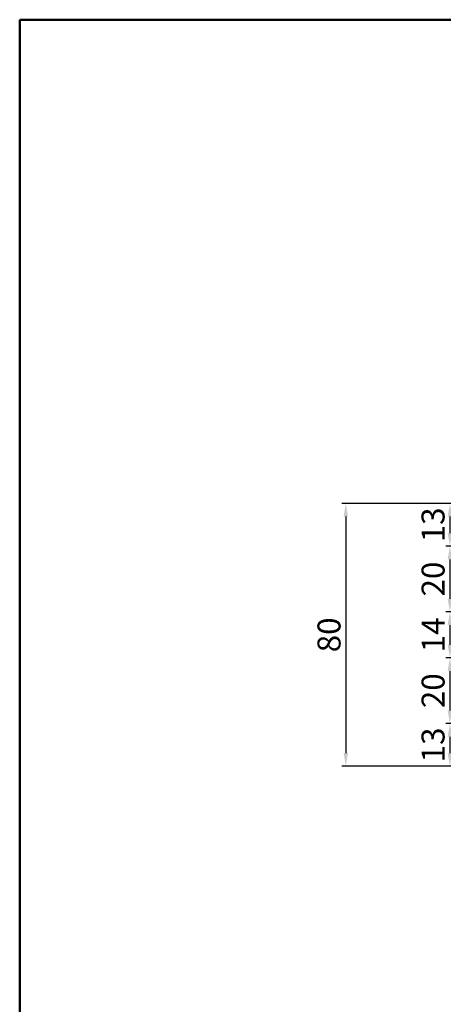
# Model space of a CAD drawing. Units: millimetres. Extents: x -21 to 693, y -570 to 295.
# Tile 3 of 7: x -21 to 107, y -4 to 295. Entities that reach past the tile are written whole.
import ezdxf

# ---------------------------------------------------------------- set-up
doc = ezdxf.new("R2010")
doc.units = ezdxf.units.MM
doc.header["$LTSCALE"] = 0.5
doc.layers.add('M-DIMS', color=2, linetype='Continuous', lineweight=25)
doc.layers.add('M-TTLB', color=7, linetype='Continuous', lineweight=50)
doc.styles.get("Standard").update_dxf_attribs({"font": 'arial.ttf'})
doc.dimstyles.new('ISO-25', dxfattribs={"dimtxt": 7, "dimasz": 4, "dimexe": 1.25, "dimexo": 0.625, "dimtad": 1, "dimdec": 0, "dimtxsty": 'Standard', "dimcen": 2.5, "dimadec": 0, "dimazin": 0, "dimtfac": 1, "dimtdec": 0, "dimtofl": 0, "dimtmove": 0, "dimatfit": 3, "dimfxl": 1, "dimarcsym": 0})

# ---------------------------------------------------------------- blocks, each defined once
blk = doc.blocks.new('*D6')
at = {"layer": 'Defpoints', "color": 0, "ltscale": 0.5, "transparency": 16777216}
for p in [(136.24, 148.11), (77.7, 68.11), (136.24, 68.11)]:
    blk.add_point(p, dxfattribs=at)
at = {"layer": 'M-DIMS', "color": 0, "lineweight": -2, "ltscale": 0.5, "transparency": 16777216}
for p, q in [((135.61, 148.11), (76.45, 148.11)), ((77.7, 144.11), (77.7, 72.11)), ((135.61, 68.11), (76.45, 68.11))]:
    blk.add_line(p, q, dxfattribs=at)
at = {"layer": 'M-DIMS', "color": 0, "ltscale": 0.5, "transparency": 16777216}
for points in [[(77.04, 144.11), (78.37, 144.11), (77.7, 148.11)], [(77.04, 72.11), (78.37, 72.11), (77.7, 68.11)]]:
    blk.add_solid(points, dxfattribs=at)
at = {"layer": 'M-DIMS', "color": 0, "ltscale": 0.5, "transparency": 16777216, "insert": (73.5, 108.11), "char_height": 7, "attachment_point": 5, "rotation": 90}
blk.add_mtext('80', dxfattribs=at)
blk = doc.blocks.new('*D7')
at = {"layer": 'Defpoints', "color": 0, "ltscale": 0.5, "transparency": 16777216}
for p in [(136.24, 148.11), (109.35, 135.11), (136.24, 135.11)]:
    blk.add_point(p, dxfattribs=at)
at = {"layer": 'M-DIMS', "color": 0, "lineweight": -2, "ltscale": 0.5, "transparency": 16777216}
for p, q in [((135.61, 148.11), (108.1, 148.11)), ((109.35, 144.11), (109.35, 139.11)), ((135.61, 135.11), (108.1, 135.11))]:
    blk.add_line(p, q, dxfattribs=at)
at = {"layer": 'M-DIMS', "color": 0, "ltscale": 0.5, "transparency": 16777216}
for points in [[(108.69, 144.11), (110.02, 144.11), (109.35, 148.11)], [(108.69, 139.11), (110.02, 139.11), (109.35, 135.11)]]:
    blk.add_solid(points, dxfattribs=at)
at = {"layer": 'M-DIMS', "color": 0, "ltscale": 0.5, "transparency": 16777216, "insert": (105.15, 141.61), "char_height": 7, "attachment_point": 5, "rotation": 90}
blk.add_mtext('13', dxfattribs=at)
blk = doc.blocks.new('*D8')
at = {"layer": 'Defpoints', "color": 0, "ltscale": 0.5, "transparency": 16777216}
for p in [(135.24, 135.11), (109.35, 115.11), (136.24, 115.11)]:
    blk.add_point(p, dxfattribs=at)
at = {"layer": 'M-DIMS', "color": 0, "lineweight": -2, "ltscale": 0.5, "transparency": 16777216}
for p, q in [((134.61, 135.11), (108.1, 135.11)), ((109.35, 131.11), (109.35, 119.11)), ((135.61, 115.11), (108.1, 115.11))]:
    blk.add_line(p, q, dxfattribs=at)
at = {"layer": 'M-DIMS', "color": 0, "ltscale": 0.5, "transparency": 16777216}
for points in [[(108.69, 131.11), (110.02, 131.11), (109.35, 135.11)], [(108.69, 119.11), (110.02, 119.11), (109.35, 115.11)]]:
    blk.add_solid(points, dxfattribs=at)
at = {"layer": 'M-DIMS', "color": 0, "ltscale": 0.5, "transparency": 16777216, "insert": (105.16, 125.11), "char_height": 7, "attachment_point": 5, "rotation": 90}
blk.add_mtext('20', dxfattribs=at)
blk = doc.blocks.new('*D9')
at = {"layer": 'Defpoints', "color": 0, "ltscale": 0.5, "transparency": 16777216}
for p in [(136.24, 115.11), (109.35, 101.11), (136.24, 101.11)]:
    blk.add_point(p, dxfattribs=at)
at = {"layer": 'M-DIMS', "color": 0, "lineweight": -2, "ltscale": 0.5, "transparency": 16777216}
for p, q in [((135.61, 115.11), (108.1, 115.11)), ((109.35, 111.11), (109.35, 105.11)), ((135.61, 101.11), (108.1, 101.11))]:
    blk.add_line(p, q, dxfattribs=at)
at = {"layer": 'M-DIMS', "color": 0, "ltscale": 0.5, "transparency": 16777216}
for points in [[(108.69, 111.11), (110.02, 111.11), (109.35, 115.11)], [(108.69, 105.11), (110.02, 105.11), (109.35, 101.11)]]:
    blk.add_solid(points, dxfattribs=at)
at = {"layer": 'M-DIMS', "color": 0, "ltscale": 0.5, "transparency": 16777216, "insert": (105.21, 108.11), "char_height": 7, "attachment_point": 5, "rotation": 90}
blk.add_mtext('14', dxfattribs=at)
blk = doc.blocks.new('*D10')
at = {"layer": 'Defpoints', "color": 0, "ltscale": 0.5, "transparency": 16777216}
for p in [(136.24, 101.11), (109.35, 81.11), (135.24, 81.11)]:
    blk.add_point(p, dxfattribs=at)
at = {"layer": 'M-DIMS', "color": 0, "lineweight": -2, "ltscale": 0.5, "transparency": 16777216}
for p, q in [((135.61, 101.11), (108.1, 101.11)), ((109.35, 97.11), (109.35, 85.11)), ((134.61, 81.11), (108.1, 81.11))]:
    blk.add_line(p, q, dxfattribs=at)
at = {"layer": 'M-DIMS', "color": 0, "ltscale": 0.5, "transparency": 16777216}
for points in [[(108.69, 97.11), (110.02, 97.11), (109.35, 101.11)], [(108.69, 85.11), (110.02, 85.11), (109.35, 81.11)]]:
    blk.add_solid(points, dxfattribs=at)
at = {"layer": 'M-DIMS', "color": 0, "ltscale": 0.5, "transparency": 16777216, "insert": (105.16, 91.11), "char_height": 7, "attachment_point": 5, "rotation": 90}
blk.add_mtext('20', dxfattribs=at)
blk = doc.blocks.new('*D11')
at = {"layer": 'Defpoints', "color": 0, "ltscale": 0.5, "transparency": 16777216}
for p in [(129.36, 81.11), (109.35, 68.11), (136.24, 68.11)]:
    blk.add_point(p, dxfattribs=at)
at = {"layer": 'M-DIMS', "color": 0, "lineweight": -2, "ltscale": 0.5, "transparency": 16777216}
for p, q in [((128.74, 81.11), (108.1, 81.11)), ((109.35, 77.11), (109.35, 72.11)), ((135.61, 68.11), (108.1, 68.11))]:
    blk.add_line(p, q, dxfattribs=at)
at = {"layer": 'M-DIMS', "color": 0, "ltscale": 0.5, "transparency": 16777216}
for points in [[(108.69, 77.11), (110.02, 77.11), (109.35, 81.11)], [(108.69, 72.11), (110.02, 72.11), (109.35, 68.11)]]:
    blk.add_solid(points, dxfattribs=at)
at = {"layer": 'M-DIMS', "color": 0, "ltscale": 0.5, "transparency": 16777216, "insert": (105.15, 74.61), "char_height": 7, "attachment_point": 5, "rotation": 90}
blk.add_mtext('13', dxfattribs=at)

msp = doc.modelspace()

# ---------------------------------------------------------------- linework, layer by layer
at = {"layer": 'M-TTLB', "ltscale": 0.5}
msp.add_lwpolyline([(-21.49, 295.4176), (693.1139, 295.4176), (693.1139, -570.0874), (-21.49, -570.0874)], close=True, dxfattribs=at)

# ---------------------------------------------------------------- dimensions: what is measured, and where the dimension line sits
at = {"layer": 'M-DIMS', "ltscale": 0.5}
for base, p1, p2, picture, middle in [((77.7017, 68.1134), (136.2368, 148.1134), (136.2368, 68.1134), '*D6', (73.5027, 108.1134)), ((109.354, 135.1134), (136.2368, 148.1134), (136.2368, 135.1134), '*D7', (105.1526, 141.6134)), ((109.354, 115.1134), (135.2368, 135.1134), (136.2368, 115.1134), '*D8', (105.155, 125.1134)), ((109.354, 101.1134), (136.2368, 115.1134), (136.2368, 101.1134), '*D9', (105.2147, 108.1134)), ((109.354, 81.1134), (136.2368, 101.1134), (135.2368, 81.1134), '*D10', (105.155, 91.1134)), ((109.354, 68.1134), (129.3604, 81.1134), (136.2368, 68.1134), '*D11', (105.1526, 74.6134))]:
    dim = msp.add_linear_dim(base=base, p1=p1, p2=p2, angle=90, dimstyle='ISO-25', override={"dimclrd": 0, "dimclre": 0, "dimclrt": 0}, dxfattribs=at)
    dim.commit()
    dim.dimension.update_dxf_attribs({"geometry": picture, "text_midpoint": middle})

doc.saveas('drawing.dxf')
